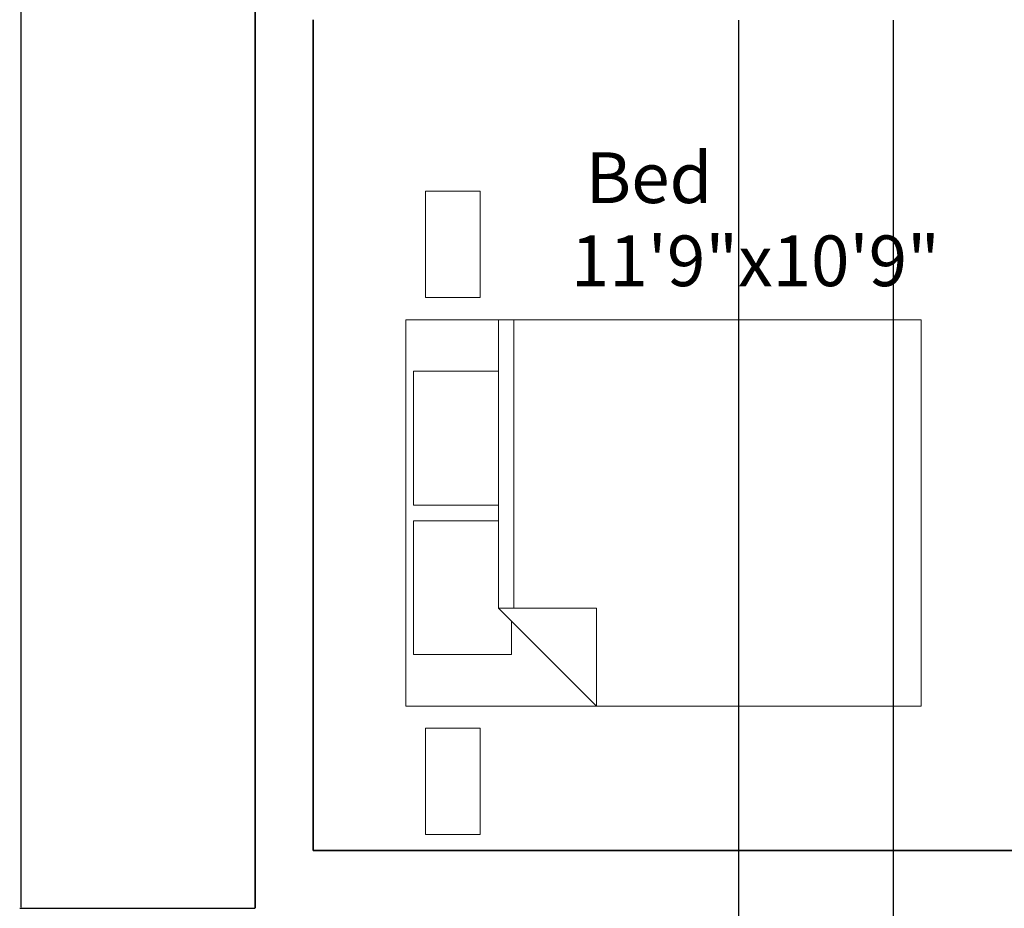
# Model space of a CAD drawing. Units: inches. Extents: x 108 to 613, y 1573 to 2319.
# Tile 2 of 11: x 108 to 261, y 1989 to 2127. Entities that reach past the tile are written whole.
import ezdxf

# ---------------------------------------------------------------- set-up
doc = ezdxf.new("R2010")
doc.units = ezdxf.units.IN
for name, color, linetype, lineweight in [('A-ANNO-DIMS', 2, 'Continuous', 18), ('A-AREA-IDEN', 3, 'Continuous', 18), ('furniture', 2, 'Continuous', 18), ('wall', 6, 'Continuous', 35)]:
    doc.layers.add(name, color=color, linetype=linetype, lineweight=lineweight)
doc.styles.get("Standard").update_dxf_attribs({"font": 'arial.ttf'})
doc.dimstyles.get("Standard").update_dxf_attribs({"dimtxt": 0.18, "dimasz": 0.18, "dimexe": 0.18, "dimexo": 0.0625, "dimgap": 0.09, "dimtad": 0, "dimtih": 1, "dimtoh": 1, "dimdec": 4, "dimzin": 0, "dimdsep": 46, "dimtxsty": 'Standard', "dimcen": 0.09, "dimadec": 0, "dimazin": 0, "dimtfac": 1, "dimtdec": 4, "dimtofl": 0, "dimtmove": 0, "dimatfit": 3, "dimfxl": 1, "dimtolj": 1, "dimtzin": 0, "dimarcsym": 0})

# ---------------------------------------------------------------- blocks, each defined once
blk = doc.blocks.new('Bed - Queen')
for p, q in [((0, -80.00003), (0, 0)), ((0, 0), (59.99999, 0)), ((59.99999, 0), (59.99999, -80.00003)), ((7.99999, -1.2), (28.79998, -1.2)), ((7.99999, -14.4), (7.99999, -1.2)), ((28.79998, -1.2), (28.79998, -14.4)), ((31.19999, -1.2), (51.99999, -1.2)), ((31.19999, -14.4), (31.19999, -1.2)), ((51.99999, -1.2), (51.99999, -16.4)), ((0, -14.4), (44.8, -14.4)), ((59.99999, -29.6), (44.8, -14.4)), ((44.8, -14.4), (44.8, -29.6)), ((44.8, -16.8), (0, -16.8)), ((51.99999, -16.4), (46.79936, -16.4)), ((44.8, -29.6), (59.99999, -29.6)), ((59.99999, -80.00003), (0, -80.00003))]:
    blk.add_line(p, q)
blk = doc.blocks.new('NIGHTSTAND')
blk.add_lwpolyline([(0, 8.48), (16.5, 8.48), (16.5, 0), (0, 0)], close=True)
blk = doc.blocks.new('*D45')
at = {"layer": 'A-ANNO-DIMS', "color": 0, "lineweight": -2, "transparency": 16777216}
for p, q in [((144.71, 2276.61), (108.25, 2276.61)), ((108.43, 2276.43), (108.43, 2132.79)), ((108.43, 1988.79), (108.43, 2132.43)), ((144.71, 1988.61), (108.25, 1988.61))]:
    blk.add_line(p, q, dxfattribs=at)
at = {"layer": 'A-ANNO-DIMS', "color": 0, "transparency": 16777216}
for points in [[(108.4, 2276.43), (108.46, 2276.43), (108.43, 2276.61)], [(108.4, 1988.79), (108.46, 1988.79), (108.43, 1988.61)]]:
    blk.add_solid(points, dxfattribs=at)
at = {"layer": 'Defpoints', "color": 0, "transparency": 16777216}
for p in [(108.43, 2276.61), (144.78, 2276.61), (144.78, 1988.61)]:
    blk.add_point(p, dxfattribs=at)
at = {"layer": 'A-ANNO-DIMS', "color": 0, "transparency": 16777216, "insert": (108.43, 2132.61), "char_height": 0.18, "attachment_point": 5}
blk.add_mtext('\\A1;288', dxfattribs=at)
blk = doc.blocks.new('*D49')
at = {"layer": 'A-ANNO-DIMS', "color": 0, "lineweight": -2, "transparency": 16777216}
for p, q in [((219.78, 2126.55), (219.78, 1583.23)), ((243.78, 2126.55), (243.78, 1583.23)), ((219.96, 1583.41), (231.56, 1583.41)), ((243.6, 1583.41), (232, 1583.41))]:
    blk.add_line(p, q, dxfattribs=at)
at = {"layer": 'A-ANNO-DIMS', "color": 0, "transparency": 16777216}
for points in [[(219.96, 1583.44), (219.96, 1583.38), (219.78, 1583.41)], [(243.6, 1583.44), (243.6, 1583.38), (243.78, 1583.41)]]:
    blk.add_solid(points, dxfattribs=at)
at = {"layer": 'Defpoints', "color": 0, "transparency": 16777216}
for p in [(219.78, 2126.61), (243.78, 2126.61), (243.78, 1583.41)]:
    blk.add_point(p, dxfattribs=at)
at = {"layer": 'A-ANNO-DIMS', "color": 0, "transparency": 16777216, "insert": (231.78, 1583.41), "char_height": 0.18, "attachment_point": 5}
blk.add_mtext('\\A1;24', dxfattribs=at)

msp = doc.modelspace()

# ---------------------------------------------------------------- linework, layer by layer
at = {"layer": 'wall'}
for p, q in [((144.7753, 2276.6125), (144.7753, 1988.6125)), ((153.7753, 2126.6125), (153.7753, 1997.6125)), ((153.7753, 1997.6125), (294.7753, 1997.6125))]:
    msp.add_line(p, q, dxfattribs=at)

# ---------------------------------------------------------------- block references
at = {"layer": 'furniture', "extrusion": (0, 0, -1), "zscale": -1}
for p, rotation in [((-179.7004, 2099.9816), 269.999999999999), ((-179.7004, 2016.5755), 269.9999999999968)]:
    msp.add_blockref('NIGHTSTAND', p, dxfattribs=dict(at, rotation=rotation))
at = {"layer": 'furniture', "xscale": -1, "rotation": 90}
msp.add_blockref('Bed - Queen', (168.1312, 2080.0117), dxfattribs=at)

# ---------------------------------------------------------------- texts
at = {"layer": 'A-AREA-IDEN'}
for s, height, p in [('Bed', 7.87346, (196.0628, 2098.1344)), ('11\'9"x10\'9"', 7.873465, (193.7544, 2085.2285))]:
    msp.add_text(s, height=height, dxfattribs=at).set_placement(p)

# ---------------------------------------------------------------- dimensions: what is measured, and where the dimension line sits
at = {"layer": 'A-ANNO-DIMS'}
dim = msp.add_linear_dim(base=(108.4253, 2276.6125), p1=(144.7753, 1988.6125), p2=(144.7753, 2276.6125), angle=90, dimstyle='Standard', override={"dimdec": 0, "dimlfac": 1, "dimrnd": 0, "dimzin": 0, "dimdsep": 46, "dimlunit": 2}, dxfattribs=at)
dim.commit()
dim.dimension.update_dxf_attribs({"geometry": '*D45', "text_midpoint": (108.4253, 2132.6125)})
dim = msp.add_linear_dim(base=(243.7753, 1583.4147), p1=(219.7753, 2126.6125), p2=(243.7753, 2126.6125), dimstyle='Standard', override={"dimdec": 0, "dimlfac": 1, "dimrnd": 0, "dimzin": 0, "dimdsep": 46, "dimlunit": 2}, dxfattribs=at)
dim.commit()
dim.dimension.update_dxf_attribs({"geometry": '*D49', "text_midpoint": (231.7753, 1583.4147)})

doc.saveas('drawing.dxf')
